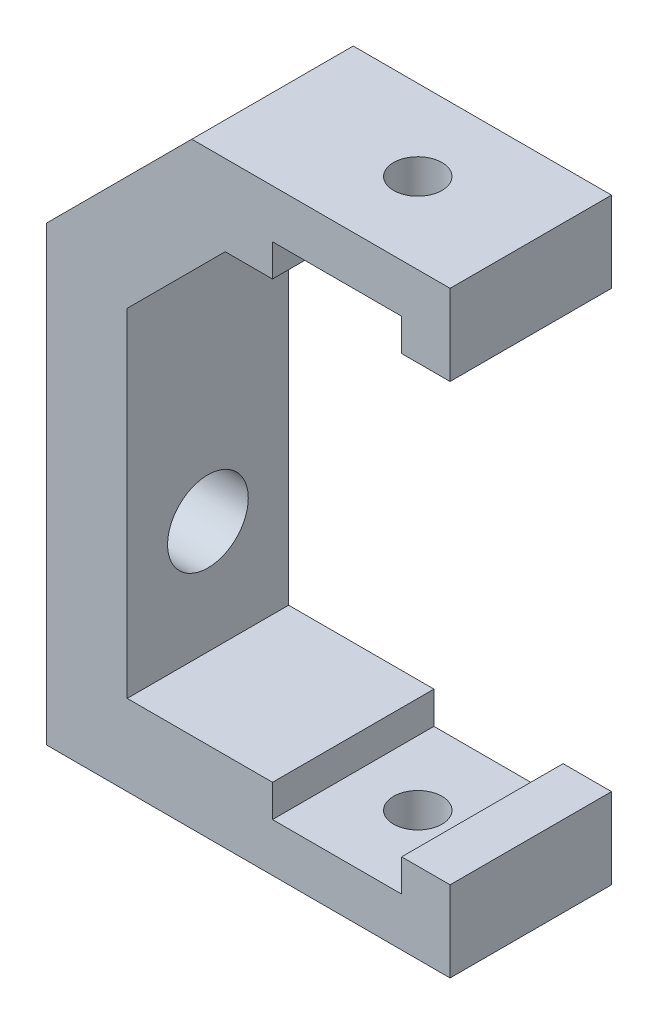
ISO-10303-21;
HEADER;
FILE_DESCRIPTION(('STEP AP214'),'2;1');
FILE_NAME('part.step','',(''),(''),'','','');
FILE_SCHEMA(('AUTOMOTIVE_DESIGN { 1 0 10303 214 1 1 1 1 }'));
ENDSEC;
DATA;
#1=APPLICATION_CONTEXT('core data for automotive mechanical design processes');
#2=APPLICATION_PROTOCOL_DEFINITION('international standard','automotive_design',2000,#1);
#3=PRODUCT_CONTEXT('',#1,'mechanical');
#4=PRODUCT('Part','Part','',(#3));
#5=PRODUCT_RELATED_PRODUCT_CATEGORY('part','',(#4));
#6=PRODUCT_DEFINITION_FORMATION('','',#4);
#7=PRODUCT_DEFINITION_CONTEXT('part definition',#1,'design');
#8=PRODUCT_DEFINITION('design','',#6,#7);
#9=PRODUCT_DEFINITION_SHAPE('','',#8);
#10=(LENGTH_UNIT() NAMED_UNIT(*) SI_UNIT(.MILLI.,.METRE.));
#11=(NAMED_UNIT(*) PLANE_ANGLE_UNIT() SI_UNIT($,.RADIAN.));
#12=(NAMED_UNIT(*) SI_UNIT($,.STERADIAN.) SOLID_ANGLE_UNIT());
#13=UNCERTAINTY_MEASURE_WITH_UNIT(LENGTH_MEASURE(1.E-05),#10,'distance_accuracy_value','');
#14=(GEOMETRIC_REPRESENTATION_CONTEXT(3) GLOBAL_UNCERTAINTY_ASSIGNED_CONTEXT((#13)) GLOBAL_UNIT_ASSIGNED_CONTEXT((#10,
#11,#12)) REPRESENTATION_CONTEXT('',''));
#15=CARTESIAN_POINT('',(0.,0.,0.));
#16=DIRECTION('',(0.,0.,1.));
#17=DIRECTION('',(1.,0.,0.));
#18=AXIS2_PLACEMENT_3D('',#15,#16,#17);
#19=CARTESIAN_POINT('',(25.,0.,5.));
#20=DIRECTION('',(0.,1.,0.));
#21=DIRECTION('',(-1.,0.,0.));
#22=AXIS2_PLACEMENT_3D('',#19,#20,#21);
#23=PLANE('',#22);
#24=CARTESIAN_POINT('',(18.,0.,0.));
#25=DIRECTION('',(0.,1.,0.));
#26=DIRECTION('',(-1.,0.,0.));
#27=AXIS2_PLACEMENT_3D('',#24,#25,#26);
#28=CIRCLE('',#27,1.5);
#29=CARTESIAN_POINT('',(16.5,0.,0.));
#30=VERTEX_POINT('',#29);
#31=EDGE_CURVE('E203',#30,#30,#28,.T.);
#32=ORIENTED_EDGE('',*,*,#31,.T.);
#33=EDGE_LOOP('',(#32));
#34=FACE_BOUND('',#33,.T.);
#35=DIRECTION('',(1.,0.,0.));
#36=VECTOR('',#35,1.);
#37=CARTESIAN_POINT('',(25.,0.,-5.));
#38=LINE('',#37,#36);
#39=CARTESIAN_POINT('',(0.,0.,-5.));
#40=VERTEX_POINT('',#39);
#41=CARTESIAN_POINT('',(25.,0.,-5.));
#42=VERTEX_POINT('',#41);
#43=EDGE_CURVE('E197',#40,#42,#38,.T.);
#44=ORIENTED_EDGE('',*,*,#43,.T.);
#45=DIRECTION('',(0.,0.,-1.));
#46=VECTOR('',#45,1.);
#47=CARTESIAN_POINT('',(25.,0.,5.));
#48=LINE('',#47,#46);
#49=CARTESIAN_POINT('',(25.,0.,5.));
#50=VERTEX_POINT('',#49);
#51=EDGE_CURVE('E11',#50,#42,#48,.T.);
#52=ORIENTED_EDGE('',*,*,#51,.F.);
#53=DIRECTION('',(1.,0.,0.));
#54=VECTOR('',#53,1.);
#55=CARTESIAN_POINT('',(25.,0.,5.));
#56=LINE('',#55,#54);
#57=CARTESIAN_POINT('',(0.,0.,5.));
#58=VERTEX_POINT('',#57);
#59=EDGE_CURVE('E232',#58,#50,#56,.T.);
#60=ORIENTED_EDGE('',*,*,#59,.F.);
#61=DIRECTION('',(0.,0.,-1.));
#62=VECTOR('',#61,1.);
#63=CARTESIAN_POINT('',(0.,0.,5.));
#64=LINE('',#63,#62);
#65=EDGE_CURVE('E194',#58,#40,#64,.T.);
#66=ORIENTED_EDGE('',*,*,#65,.T.);
#67=EDGE_LOOP('',(#44,#52,#60,#66));
#68=FACE_BOUND('',#67,.T.);
#69=ADVANCED_FACE('F39',(#34,#68),#23,.F.);
#70=CARTESIAN_POINT('',(25.,5.,5.));
#71=DIRECTION('',(-1.,0.,0.));
#72=DIRECTION('',(0.,-1.,0.));
#73=AXIS2_PLACEMENT_3D('',#70,#71,#72);
#74=PLANE('',#73);
#75=DIRECTION('',(0.,1.,0.));
#76=VECTOR('',#75,1.);
#77=CARTESIAN_POINT('',(25.,5.,-5.));
#78=LINE('',#77,#76);
#79=CARTESIAN_POINT('',(25.,5.,-5.));
#80=VERTEX_POINT('',#79);
#81=EDGE_CURVE('E199',#42,#80,#78,.T.);
#82=ORIENTED_EDGE('',*,*,#81,.T.);
#83=DIRECTION('',(0.,0.,-1.));
#84=VECTOR('',#83,1.);
#85=CARTESIAN_POINT('',(25.,5.,5.));
#86=LINE('',#85,#84);
#87=CARTESIAN_POINT('',(25.,5.,5.));
#88=VERTEX_POINT('',#87);
#89=EDGE_CURVE('E48',#88,#80,#86,.T.);
#90=ORIENTED_EDGE('',*,*,#89,.F.);
#91=DIRECTION('',(0.,1.,0.));
#92=VECTOR('',#91,1.);
#93=CARTESIAN_POINT('',(25.,5.,5.));
#94=LINE('',#93,#92);
#95=EDGE_CURVE('E128',#50,#88,#94,.T.);
#96=ORIENTED_EDGE('',*,*,#95,.F.);
#97=ORIENTED_EDGE('',*,*,#51,.T.);
#98=EDGE_LOOP('',(#82,#90,#96,#97));
#99=FACE_BOUND('',#98,.T.);
#100=ADVANCED_FACE('F346',(#99),#74,.F.);
#101=CARTESIAN_POINT('',(22.,5.,5.));
#102=DIRECTION('',(0.,-1.,0.));
#103=DIRECTION('',(0.,0.,-1.));
#104=AXIS2_PLACEMENT_3D('',#101,#102,#103);
#105=PLANE('',#104);
#106=DIRECTION('',(-1.,0.,0.));
#107=VECTOR('',#106,1.);
#108=CARTESIAN_POINT('',(22.,5.,-5.));
#109=LINE('',#108,#107);
#110=CARTESIAN_POINT('',(22.,5.,-5.));
#111=VERTEX_POINT('',#110);
#112=EDGE_CURVE('E201',#80,#111,#109,.T.);
#113=ORIENTED_EDGE('',*,*,#112,.T.);
#114=DIRECTION('',(0.,0.,-1.));
#115=VECTOR('',#114,1.);
#116=CARTESIAN_POINT('',(22.,5.,5.));
#117=LINE('',#116,#115);
#118=CARTESIAN_POINT('',(22.,5.,5.));
#119=VERTEX_POINT('',#118);
#120=EDGE_CURVE('E267',#119,#111,#117,.T.);
#121=ORIENTED_EDGE('',*,*,#120,.F.);
#122=DIRECTION('',(-1.,0.,0.));
#123=VECTOR('',#122,1.);
#124=CARTESIAN_POINT('',(22.,5.,5.));
#125=LINE('',#124,#123);
#126=EDGE_CURVE('E294',#88,#119,#125,.T.);
#127=ORIENTED_EDGE('',*,*,#126,.F.);
#128=ORIENTED_EDGE('',*,*,#89,.T.);
#129=EDGE_LOOP('',(#113,#121,#127,#128));
#130=FACE_BOUND('',#129,.T.);
#131=ADVANCED_FACE('F351',(#130),#105,.F.);
#132=CARTESIAN_POINT('',(22.,3.,5.));
#133=DIRECTION('',(1.,0.,0.));
#134=DIRECTION('',(0.,0.,-1.));
#135=AXIS2_PLACEMENT_3D('',#132,#133,#134);
#136=PLANE('',#135);
#137=DIRECTION('',(0.,-1.,0.));
#138=VECTOR('',#137,1.);
#139=CARTESIAN_POINT('',(22.,3.,-5.));
#140=LINE('',#139,#138);
#141=CARTESIAN_POINT('',(22.,3.,-5.));
#142=VERTEX_POINT('',#141);
#143=EDGE_CURVE('E202',#111,#142,#140,.T.);
#144=ORIENTED_EDGE('',*,*,#143,.T.);
#145=DIRECTION('',(0.,0.,-1.));
#146=VECTOR('',#145,1.);
#147=CARTESIAN_POINT('',(22.,3.,5.));
#148=LINE('',#147,#146);
#149=CARTESIAN_POINT('',(22.,3.,5.));
#150=VERTEX_POINT('',#149);
#151=EDGE_CURVE('E266',#150,#142,#148,.T.);
#152=ORIENTED_EDGE('',*,*,#151,.F.);
#153=DIRECTION('',(0.,-1.,0.));
#154=VECTOR('',#153,1.);
#155=CARTESIAN_POINT('',(22.,3.,5.));
#156=LINE('',#155,#154);
#157=EDGE_CURVE('E298',#119,#150,#156,.T.);
#158=ORIENTED_EDGE('',*,*,#157,.F.);
#159=ORIENTED_EDGE('',*,*,#120,.T.);
#160=EDGE_LOOP('',(#144,#152,#158,#159));
#161=FACE_BOUND('',#160,.T.);
#162=ADVANCED_FACE('F462',(#161),#136,.F.);
#163=CARTESIAN_POINT('',(14.,3.,5.));
#164=DIRECTION('',(0.,-1.,0.));
#165=DIRECTION('',(0.,0.,-1.));
#166=AXIS2_PLACEMENT_3D('',#163,#164,#165);
#167=PLANE('',#166);
#168=CARTESIAN_POINT('',(18.,3.,0.));
#169=DIRECTION('',(0.,-1.,0.));
#170=DIRECTION('',(0.,0.,-1.));
#171=AXIS2_PLACEMENT_3D('',#168,#169,#170);
#172=CIRCLE('',#171,1.5);
#173=CARTESIAN_POINT('',(18.,3.,-1.5));
#174=VERTEX_POINT('',#173);
#175=EDGE_CURVE('E278',#174,#174,#172,.T.);
#176=ORIENTED_EDGE('',*,*,#175,.T.);
#177=EDGE_LOOP('',(#176));
#178=FACE_BOUND('',#177,.T.);
#179=DIRECTION('',(-1.,0.,0.));
#180=VECTOR('',#179,1.);
#181=CARTESIAN_POINT('',(14.,3.,-5.));
#182=LINE('',#181,#180);
#183=CARTESIAN_POINT('',(14.,3.,-5.));
#184=VERTEX_POINT('',#183);
#185=EDGE_CURVE('E210',#142,#184,#182,.T.);
#186=ORIENTED_EDGE('',*,*,#185,.T.);
#187=DIRECTION('',(0.,0.,-1.));
#188=VECTOR('',#187,1.);
#189=CARTESIAN_POINT('',(14.,3.,5.));
#190=LINE('',#189,#188);
#191=CARTESIAN_POINT('',(14.,3.,5.));
#192=VERTEX_POINT('',#191);
#193=EDGE_CURVE('E263',#192,#184,#190,.T.);
#194=ORIENTED_EDGE('',*,*,#193,.F.);
#195=DIRECTION('',(-1.,0.,0.));
#196=VECTOR('',#195,1.);
#197=CARTESIAN_POINT('',(14.,3.,5.));
#198=LINE('',#197,#196);
#199=EDGE_CURVE('E297',#150,#192,#198,.T.);
#200=ORIENTED_EDGE('',*,*,#199,.F.);
#201=ORIENTED_EDGE('',*,*,#151,.T.);
#202=EDGE_LOOP('',(#186,#194,#200,#201));
#203=FACE_BOUND('',#202,.T.);
#204=ADVANCED_FACE('F457',(#178,#203),#167,.F.);
#205=CARTESIAN_POINT('',(14.,5.,5.));
#206=DIRECTION('',(-1.,0.,0.));
#207=DIRECTION('',(0.,0.,1.));
#208=AXIS2_PLACEMENT_3D('',#205,#206,#207);
#209=PLANE('',#208);
#210=DIRECTION('',(0.,1.,0.));
#211=VECTOR('',#210,1.);
#212=CARTESIAN_POINT('',(14.,5.,-5.));
#213=LINE('',#212,#211);
#214=CARTESIAN_POINT('',(14.,5.,-5.));
#215=VERTEX_POINT('',#214);
#216=EDGE_CURVE('E207',#184,#215,#213,.T.);
#217=ORIENTED_EDGE('',*,*,#216,.T.);
#218=DIRECTION('',(0.,0.,-1.));
#219=VECTOR('',#218,1.);
#220=CARTESIAN_POINT('',(14.,5.,5.));
#221=LINE('',#220,#219);
#222=CARTESIAN_POINT('',(14.,5.,5.));
#223=VERTEX_POINT('',#222);
#224=EDGE_CURVE('E257',#223,#215,#221,.T.);
#225=ORIENTED_EDGE('',*,*,#224,.F.);
#226=DIRECTION('',(0.,1.,0.));
#227=VECTOR('',#226,1.);
#228=CARTESIAN_POINT('',(14.,5.,5.));
#229=LINE('',#228,#227);
#230=EDGE_CURVE('E296',#192,#223,#229,.T.);
#231=ORIENTED_EDGE('',*,*,#230,.F.);
#232=ORIENTED_EDGE('',*,*,#193,.T.);
#233=EDGE_LOOP('',(#217,#225,#231,#232));
#234=FACE_BOUND('',#233,.T.);
#235=ADVANCED_FACE('F449',(#234),#209,.F.);
#236=CARTESIAN_POINT('',(5.,5.,5.));
#237=DIRECTION('',(0.,-1.,0.));
#238=DIRECTION('',(0.,0.,-1.));
#239=AXIS2_PLACEMENT_3D('',#236,#237,#238);
#240=PLANE('',#239);
#241=DIRECTION('',(-1.,0.,0.));
#242=VECTOR('',#241,1.);
#243=CARTESIAN_POINT('',(5.,5.,-5.));
#244=LINE('',#243,#242);
#245=CARTESIAN_POINT('',(5.,5.,-5.));
#246=VERTEX_POINT('',#245);
#247=EDGE_CURVE('E211',#215,#246,#244,.T.);
#248=ORIENTED_EDGE('',*,*,#247,.T.);
#249=DIRECTION('',(0.,0.,-1.));
#250=VECTOR('',#249,1.);
#251=CARTESIAN_POINT('',(5.,5.,5.));
#252=LINE('',#251,#250);
#253=CARTESIAN_POINT('',(5.,5.,5.));
#254=VERTEX_POINT('',#253);
#255=EDGE_CURVE('E260',#254,#246,#252,.T.);
#256=ORIENTED_EDGE('',*,*,#255,.F.);
#257=DIRECTION('',(-1.,0.,0.));
#258=VECTOR('',#257,1.);
#259=CARTESIAN_POINT('',(5.,5.,5.));
#260=LINE('',#259,#258);
#261=EDGE_CURVE('E302',#223,#254,#260,.T.);
#262=ORIENTED_EDGE('',*,*,#261,.F.);
#263=ORIENTED_EDGE('',*,*,#224,.T.);
#264=EDGE_LOOP('',(#248,#256,#262,#263));
#265=FACE_BOUND('',#264,.T.);
#266=ADVANCED_FACE('F444',(#265),#240,.F.);
#267=CARTESIAN_POINT('',(5.,25.9289321881346,5.));
#268=DIRECTION('',(-1.,0.,0.));
#269=DIRECTION('',(0.,-1.,0.));
#270=AXIS2_PLACEMENT_3D('',#267,#268,#269);
#271=PLANE('',#270);
#272=CARTESIAN_POINT('',(5.,12.,0.));
#273=DIRECTION('',(-1.,0.,0.));
#274=DIRECTION('',(0.,-1.,0.));
#275=AXIS2_PLACEMENT_3D('',#272,#273,#274);
#276=CIRCLE('',#275,2.5);
#277=CARTESIAN_POINT('',(5.,9.5,0.));
#278=VERTEX_POINT('',#277);
#279=EDGE_CURVE('E277',#278,#278,#276,.T.);
#280=ORIENTED_EDGE('',*,*,#279,.T.);
#281=EDGE_LOOP('',(#280));
#282=FACE_BOUND('',#281,.T.);
#283=DIRECTION('',(0.,1.,0.));
#284=VECTOR('',#283,1.);
#285=CARTESIAN_POINT('',(5.,25.9289321881346,-5.));
#286=LINE('',#285,#284);
#287=CARTESIAN_POINT('',(5.,25.9289321881346,-5.));
#288=VERTEX_POINT('',#287);
#289=EDGE_CURVE('E213',#246,#288,#286,.T.);
#290=ORIENTED_EDGE('',*,*,#289,.T.);
#291=DIRECTION('',(0.,0.,-1.));
#292=VECTOR('',#291,1.);
#293=CARTESIAN_POINT('',(5.,25.9289321881346,5.));
#294=LINE('',#293,#292);
#295=CARTESIAN_POINT('',(5.,25.9289321881346,5.));
#296=VERTEX_POINT('',#295);
#297=EDGE_CURVE('E255',#296,#288,#294,.T.);
#298=ORIENTED_EDGE('',*,*,#297,.F.);
#299=DIRECTION('',(0.,1.,0.));
#300=VECTOR('',#299,1.);
#301=CARTESIAN_POINT('',(5.,25.9289321881346,5.));
#302=LINE('',#301,#300);
#303=EDGE_CURVE('E303',#254,#296,#302,.T.);
#304=ORIENTED_EDGE('',*,*,#303,.F.);
#305=ORIENTED_EDGE('',*,*,#255,.T.);
#306=EDGE_LOOP('',(#290,#298,#304,#305));
#307=FACE_BOUND('',#306,.T.);
#308=ADVANCED_FACE('F436',(#282,#307),#271,.F.);
#309=CARTESIAN_POINT('',(11.0710678118653,32.,5.));
#310=DIRECTION('',(-0.707106781186556,0.707106781186539,0.));
#311=DIRECTION('',(-0.707106781186539,-0.707106781186556,0.));
#312=AXIS2_PLACEMENT_3D('',#309,#310,#311);
#313=PLANE('',#312);
#314=DIRECTION('',(0.707106781186539,0.707106781186556,0.));
#315=VECTOR('',#314,1.);
#316=CARTESIAN_POINT('',(11.0710678118653,32.,-5.));
#317=LINE('',#316,#315);
#318=CARTESIAN_POINT('',(11.0710678118653,32.,-5.));
#319=VERTEX_POINT('',#318);
#320=EDGE_CURVE('E214',#288,#319,#317,.T.);
#321=ORIENTED_EDGE('',*,*,#320,.T.);
#322=DIRECTION('',(0.,0.,-1.));
#323=VECTOR('',#322,1.);
#324=CARTESIAN_POINT('',(11.0710678118653,32.,5.));
#325=LINE('',#324,#323);
#326=CARTESIAN_POINT('',(11.0710678118653,32.,5.));
#327=VERTEX_POINT('',#326);
#328=EDGE_CURVE('E253',#327,#319,#325,.T.);
#329=ORIENTED_EDGE('',*,*,#328,.F.);
#330=DIRECTION('',(0.707106781186539,0.707106781186556,0.));
#331=VECTOR('',#330,1.);
#332=CARTESIAN_POINT('',(11.0710678118653,32.,5.));
#333=LINE('',#332,#331);
#334=EDGE_CURVE('E308',#296,#327,#333,.T.);
#335=ORIENTED_EDGE('',*,*,#334,.F.);
#336=ORIENTED_EDGE('',*,*,#297,.T.);
#337=EDGE_LOOP('',(#321,#329,#335,#336));
#338=FACE_BOUND('',#337,.T.);
#339=ADVANCED_FACE('F430',(#338),#313,.F.);
#340=CARTESIAN_POINT('',(14.,32.,5.));
#341=DIRECTION('',(0.,1.,0.));
#342=DIRECTION('',(0.,0.,1.));
#343=AXIS2_PLACEMENT_3D('',#340,#341,#342);
#344=PLANE('',#343);
#345=DIRECTION('',(1.,0.,0.));
#346=VECTOR('',#345,1.);
#347=CARTESIAN_POINT('',(14.,32.,-5.));
#348=LINE('',#347,#346);
#349=CARTESIAN_POINT('',(14.,32.,-5.));
#350=VERTEX_POINT('',#349);
#351=EDGE_CURVE('E220',#319,#350,#348,.T.);
#352=ORIENTED_EDGE('',*,*,#351,.T.);
#353=DIRECTION('',(0.,0.,-1.));
#354=VECTOR('',#353,1.);
#355=CARTESIAN_POINT('',(14.,32.,5.));
#356=LINE('',#355,#354);
#357=CARTESIAN_POINT('',(14.,32.,5.));
#358=VERTEX_POINT('',#357);
#359=EDGE_CURVE('E249',#358,#350,#356,.T.);
#360=ORIENTED_EDGE('',*,*,#359,.F.);
#361=DIRECTION('',(1.,0.,0.));
#362=VECTOR('',#361,1.);
#363=CARTESIAN_POINT('',(14.,32.,5.));
#364=LINE('',#363,#362);
#365=EDGE_CURVE('E306',#327,#358,#364,.T.);
#366=ORIENTED_EDGE('',*,*,#365,.F.);
#367=ORIENTED_EDGE('',*,*,#328,.T.);
#368=EDGE_LOOP('',(#352,#360,#366,#367));
#369=FACE_BOUND('',#368,.T.);
#370=ADVANCED_FACE('F416',(#369),#344,.F.);
#371=CARTESIAN_POINT('',(14.,34.,5.));
#372=DIRECTION('',(-1.,0.,0.));
#373=DIRECTION('',(0.,0.,1.));
#374=AXIS2_PLACEMENT_3D('',#371,#372,#373);
#375=PLANE('',#374);
#376=DIRECTION('',(0.,1.,0.));
#377=VECTOR('',#376,1.);
#378=CARTESIAN_POINT('',(14.,34.,-5.));
#379=LINE('',#378,#377);
#380=CARTESIAN_POINT('',(14.,34.,-5.));
#381=VERTEX_POINT('',#380);
#382=EDGE_CURVE('E218',#350,#381,#379,.T.);
#383=ORIENTED_EDGE('',*,*,#382,.T.);
#384=DIRECTION('',(0.,0.,-1.));
#385=VECTOR('',#384,1.);
#386=CARTESIAN_POINT('',(14.,34.,5.));
#387=LINE('',#386,#385);
#388=CARTESIAN_POINT('',(14.,34.,5.));
#389=VERTEX_POINT('',#388);
#390=EDGE_CURVE('E241',#389,#381,#387,.T.);
#391=ORIENTED_EDGE('',*,*,#390,.F.);
#392=DIRECTION('',(0.,1.,0.));
#393=VECTOR('',#392,1.);
#394=CARTESIAN_POINT('',(14.,34.,5.));
#395=LINE('',#394,#393);
#396=EDGE_CURVE('E309',#358,#389,#395,.T.);
#397=ORIENTED_EDGE('',*,*,#396,.F.);
#398=ORIENTED_EDGE('',*,*,#359,.T.);
#399=EDGE_LOOP('',(#383,#391,#397,#398));
#400=FACE_BOUND('',#399,.T.);
#401=ADVANCED_FACE('F413',(#400),#375,.F.);
#402=CARTESIAN_POINT('',(22.,34.,5.));
#403=DIRECTION('',(0.,1.,0.));
#404=DIRECTION('',(-1.,0.,0.));
#405=AXIS2_PLACEMENT_3D('',#402,#403,#404);
#406=PLANE('',#405);
#407=CARTESIAN_POINT('',(18.,34.,0.));
#408=DIRECTION('',(0.,1.,0.));
#409=DIRECTION('',(-1.,0.,0.));
#410=AXIS2_PLACEMENT_3D('',#407,#408,#409);
#411=CIRCLE('',#410,1.5);
#412=CARTESIAN_POINT('',(16.5,34.,0.));
#413=VERTEX_POINT('',#412);
#414=EDGE_CURVE('E274',#413,#413,#411,.T.);
#415=ORIENTED_EDGE('',*,*,#414,.T.);
#416=EDGE_LOOP('',(#415));
#417=FACE_BOUND('',#416,.T.);
#418=DIRECTION('',(1.,0.,0.));
#419=VECTOR('',#418,1.);
#420=CARTESIAN_POINT('',(22.,34.,-5.));
#421=LINE('',#420,#419);
#422=CARTESIAN_POINT('',(22.,34.,-5.));
#423=VERTEX_POINT('',#422);
#424=EDGE_CURVE('E222',#381,#423,#421,.T.);
#425=ORIENTED_EDGE('',*,*,#424,.T.);
#426=DIRECTION('',(0.,0.,-1.));
#427=VECTOR('',#426,1.);
#428=CARTESIAN_POINT('',(22.,34.,5.));
#429=LINE('',#428,#427);
#430=CARTESIAN_POINT('',(22.,34.,5.));
#431=VERTEX_POINT('',#430);
#432=EDGE_CURVE('E244',#431,#423,#429,.T.);
#433=ORIENTED_EDGE('',*,*,#432,.F.);
#434=DIRECTION('',(1.,0.,0.));
#435=VECTOR('',#434,1.);
#436=CARTESIAN_POINT('',(22.,34.,5.));
#437=LINE('',#436,#435);
#438=EDGE_CURVE('E315',#389,#431,#437,.T.);
#439=ORIENTED_EDGE('',*,*,#438,.F.);
#440=ORIENTED_EDGE('',*,*,#390,.T.);
#441=EDGE_LOOP('',(#425,#433,#439,#440));
#442=FACE_BOUND('',#441,.T.);
#443=ADVANCED_FACE('F409',(#417,#442),#406,.F.);
#444=CARTESIAN_POINT('',(22.,32.,5.));
#445=DIRECTION('',(1.,0.,0.));
#446=DIRECTION('',(0.,1.,0.));
#447=AXIS2_PLACEMENT_3D('',#444,#445,#446);
#448=PLANE('',#447);
#449=DIRECTION('',(0.,-1.,0.));
#450=VECTOR('',#449,1.);
#451=CARTESIAN_POINT('',(22.,32.,-5.));
#452=LINE('',#451,#450);
#453=CARTESIAN_POINT('',(22.,32.,-5.));
#454=VERTEX_POINT('',#453);
#455=EDGE_CURVE('E224',#423,#454,#452,.T.);
#456=ORIENTED_EDGE('',*,*,#455,.T.);
#457=DIRECTION('',(0.,0.,-1.));
#458=VECTOR('',#457,1.);
#459=CARTESIAN_POINT('',(22.,32.,5.));
#460=LINE('',#459,#458);
#461=CARTESIAN_POINT('',(22.,32.,5.));
#462=VERTEX_POINT('',#461);
#463=EDGE_CURVE('E239',#462,#454,#460,.T.);
#464=ORIENTED_EDGE('',*,*,#463,.F.);
#465=DIRECTION('',(0.,-1.,0.));
#466=VECTOR('',#465,1.);
#467=CARTESIAN_POINT('',(22.,32.,5.));
#468=LINE('',#467,#466);
#469=EDGE_CURVE('E314',#431,#462,#468,.T.);
#470=ORIENTED_EDGE('',*,*,#469,.F.);
#471=ORIENTED_EDGE('',*,*,#432,.T.);
#472=EDGE_LOOP('',(#456,#464,#470,#471));
#473=FACE_BOUND('',#472,.T.);
#474=ADVANCED_FACE('F398',(#473),#448,.F.);
#475=CARTESIAN_POINT('',(25.,32.,5.));
#476=DIRECTION('',(0.,1.,0.));
#477=DIRECTION('',(0.,0.,1.));
#478=AXIS2_PLACEMENT_3D('',#475,#476,#477);
#479=PLANE('',#478);
#480=DIRECTION('',(1.,0.,0.));
#481=VECTOR('',#480,1.);
#482=CARTESIAN_POINT('',(25.,32.,-5.));
#483=LINE('',#482,#481);
#484=CARTESIAN_POINT('',(25.,32.,-5.));
#485=VERTEX_POINT('',#484);
#486=EDGE_CURVE('E223',#454,#485,#483,.T.);
#487=ORIENTED_EDGE('',*,*,#486,.T.);
#488=DIRECTION('',(0.,0.,-1.));
#489=VECTOR('',#488,1.);
#490=CARTESIAN_POINT('',(25.,32.,5.));
#491=LINE('',#490,#489);
#492=CARTESIAN_POINT('',(25.,32.,5.));
#493=VERTEX_POINT('',#492);
#494=EDGE_CURVE('E237',#493,#485,#491,.T.);
#495=ORIENTED_EDGE('',*,*,#494,.F.);
#496=DIRECTION('',(1.,0.,0.));
#497=VECTOR('',#496,1.);
#498=CARTESIAN_POINT('',(25.,32.,5.));
#499=LINE('',#498,#497);
#500=EDGE_CURVE('E316',#462,#493,#499,.T.);
#501=ORIENTED_EDGE('',*,*,#500,.F.);
#502=ORIENTED_EDGE('',*,*,#463,.T.);
#503=EDGE_LOOP('',(#487,#495,#501,#502));
#504=FACE_BOUND('',#503,.T.);
#505=ADVANCED_FACE('F325',(#504),#479,.F.);
#506=CARTESIAN_POINT('',(25.,37.,5.));
#507=DIRECTION('',(-1.,0.,0.));
#508=DIRECTION('',(0.,-1.,0.));
#509=AXIS2_PLACEMENT_3D('',#506,#507,#508);
#510=PLANE('',#509);
#511=DIRECTION('',(0.,1.,0.));
#512=VECTOR('',#511,1.);
#513=CARTESIAN_POINT('',(25.,37.,-5.));
#514=LINE('',#513,#512);
#515=CARTESIAN_POINT('',(25.,37.,-5.));
#516=VERTEX_POINT('',#515);
#517=EDGE_CURVE('E229',#485,#516,#514,.T.);
#518=ORIENTED_EDGE('',*,*,#517,.T.);
#519=DIRECTION('',(0.,0.,-1.));
#520=VECTOR('',#519,1.);
#521=CARTESIAN_POINT('',(25.,37.,5.));
#522=LINE('',#521,#520);
#523=CARTESIAN_POINT('',(25.,37.,5.));
#524=VERTEX_POINT('',#523);
#525=EDGE_CURVE('E187',#524,#516,#522,.T.);
#526=ORIENTED_EDGE('',*,*,#525,.F.);
#527=DIRECTION('',(0.,1.,0.));
#528=VECTOR('',#527,1.);
#529=CARTESIAN_POINT('',(25.,37.,5.));
#530=LINE('',#529,#528);
#531=EDGE_CURVE('E178',#493,#524,#530,.T.);
#532=ORIENTED_EDGE('',*,*,#531,.F.);
#533=ORIENTED_EDGE('',*,*,#494,.T.);
#534=EDGE_LOOP('',(#518,#526,#532,#533));
#535=FACE_BOUND('',#534,.T.);
#536=ADVANCED_FACE('F326',(#535),#510,.F.);
#537=CARTESIAN_POINT('',(8.99999999999977,37.,5.));
#538=DIRECTION('',(0.,-1.,0.));
#539=DIRECTION('',(0.,0.,-1.));
#540=AXIS2_PLACEMENT_3D('',#537,#538,#539);
#541=PLANE('',#540);
#542=CARTESIAN_POINT('',(18.,37.,0.));
#543=DIRECTION('',(0.,-1.,0.));
#544=DIRECTION('',(0.,0.,-1.));
#545=AXIS2_PLACEMENT_3D('',#542,#543,#544);
#546=CIRCLE('',#545,1.5);
#547=CARTESIAN_POINT('',(18.,37.,-1.5));
#548=VERTEX_POINT('',#547);
#549=EDGE_CURVE('E272',#548,#548,#546,.T.);
#550=ORIENTED_EDGE('',*,*,#549,.T.);
#551=EDGE_LOOP('',(#550));
#552=FACE_BOUND('',#551,.T.);
#553=DIRECTION('',(-1.,0.,0.));
#554=VECTOR('',#553,1.);
#555=CARTESIAN_POINT('',(8.99999999999977,37.,-5.));
#556=LINE('',#555,#554);
#557=CARTESIAN_POINT('',(8.99999999999977,37.,-5.));
#558=VERTEX_POINT('',#557);
#559=EDGE_CURVE('E189',#516,#558,#556,.T.);
#560=ORIENTED_EDGE('',*,*,#559,.T.);
#561=DIRECTION('',(0.,0.,-1.));
#562=VECTOR('',#561,1.);
#563=CARTESIAN_POINT('',(8.99999999999977,37.,5.));
#564=LINE('',#563,#562);
#565=CARTESIAN_POINT('',(8.99999999999977,37.,5.));
#566=VERTEX_POINT('',#565);
#567=EDGE_CURVE('E184',#566,#558,#564,.T.);
#568=ORIENTED_EDGE('',*,*,#567,.F.);
#569=DIRECTION('',(-1.,0.,0.));
#570=VECTOR('',#569,1.);
#571=CARTESIAN_POINT('',(8.99999999999977,37.,5.));
#572=LINE('',#571,#570);
#573=EDGE_CURVE('E172',#524,#566,#572,.T.);
#574=ORIENTED_EDGE('',*,*,#573,.F.);
#575=ORIENTED_EDGE('',*,*,#525,.T.);
#576=EDGE_LOOP('',(#560,#568,#574,#575));
#577=FACE_BOUND('',#576,.T.);
#578=ADVANCED_FACE('F183',(#552,#577),#541,.F.);
#579=CARTESIAN_POINT('',(0.,28.,5.));
#580=DIRECTION('',(0.707106781186556,-0.707106781186539,0.));
#581=DIRECTION('',(0.707106781186539,0.707106781186556,0.));
#582=AXIS2_PLACEMENT_3D('',#579,#580,#581);
#583=PLANE('',#582);
#584=DIRECTION('',(-0.707106781186539,-0.707106781186556,0.));
#585=VECTOR('',#584,1.);
#586=CARTESIAN_POINT('',(0.,28.,-5.));
#587=LINE('',#586,#585);
#588=CARTESIAN_POINT('',(0.,28.,-5.));
#589=VERTEX_POINT('',#588);
#590=EDGE_CURVE('E118',#558,#589,#587,.T.);
#591=ORIENTED_EDGE('',*,*,#590,.T.);
#592=DIRECTION('',(0.,0.,-1.));
#593=VECTOR('',#592,1.);
#594=CARTESIAN_POINT('',(0.,28.,5.));
#595=LINE('',#594,#593);
#596=CARTESIAN_POINT('',(0.,28.,5.));
#597=VERTEX_POINT('',#596);
#598=EDGE_CURVE('E190',#597,#589,#595,.T.);
#599=ORIENTED_EDGE('',*,*,#598,.F.);
#600=DIRECTION('',(-0.707106781186539,-0.707106781186556,0.));
#601=VECTOR('',#600,1.);
#602=CARTESIAN_POINT('',(0.,28.,5.));
#603=LINE('',#602,#601);
#604=EDGE_CURVE('E177',#566,#597,#603,.T.);
#605=ORIENTED_EDGE('',*,*,#604,.F.);
#606=ORIENTED_EDGE('',*,*,#567,.T.);
#607=EDGE_LOOP('',(#591,#599,#605,#606));
#608=FACE_BOUND('',#607,.T.);
#609=ADVANCED_FACE('F191',(#608),#583,.F.);
#610=CARTESIAN_POINT('',(0.,0.,5.));
#611=DIRECTION('',(1.,0.,0.));
#612=DIRECTION('',(0.,0.,-1.));
#613=AXIS2_PLACEMENT_3D('',#610,#611,#612);
#614=PLANE('',#613);
#615=CARTESIAN_POINT('',(0.,12.,0.));
#616=DIRECTION('',(1.,0.,0.));
#617=DIRECTION('',(0.,0.,-1.));
#618=AXIS2_PLACEMENT_3D('',#615,#616,#617);
#619=CIRCLE('',#618,2.5);
#620=CARTESIAN_POINT('',(0.,12.,-2.5));
#621=VERTEX_POINT('',#620);
#622=EDGE_CURVE('E45',#621,#621,#619,.T.);
#623=ORIENTED_EDGE('',*,*,#622,.T.);
#624=EDGE_LOOP('',(#623));
#625=FACE_BOUND('',#624,.T.);
#626=DIRECTION('',(0.,-1.,0.));
#627=VECTOR('',#626,1.);
#628=CARTESIAN_POINT('',(0.,0.,-5.));
#629=LINE('',#628,#627);
#630=EDGE_CURVE('E122',#589,#40,#629,.T.);
#631=ORIENTED_EDGE('',*,*,#630,.T.);
#632=ORIENTED_EDGE('',*,*,#65,.F.);
#633=DIRECTION('',(0.,-1.,0.));
#634=VECTOR('',#633,1.);
#635=CARTESIAN_POINT('',(0.,0.,5.));
#636=LINE('',#635,#634);
#637=EDGE_CURVE('E60',#597,#58,#636,.T.);
#638=ORIENTED_EDGE('',*,*,#637,.F.);
#639=ORIENTED_EDGE('',*,*,#598,.T.);
#640=EDGE_LOOP('',(#631,#632,#638,#639));
#641=FACE_BOUND('',#640,.T.);
#642=ADVANCED_FACE('F331',(#625,#641),#614,.F.);
#643=CARTESIAN_POINT('',(0.,0.,5.));
#644=DIRECTION('',(0.,0.,-1.));
#645=DIRECTION('',(-1.,0.,0.));
#646=AXIS2_PLACEMENT_3D('',#643,#644,#645);
#647=PLANE('',#646);
#648=ORIENTED_EDGE('',*,*,#59,.T.);
#649=ORIENTED_EDGE('',*,*,#95,.T.);
#650=ORIENTED_EDGE('',*,*,#126,.T.);
#651=ORIENTED_EDGE('',*,*,#157,.T.);
#652=ORIENTED_EDGE('',*,*,#199,.T.);
#653=ORIENTED_EDGE('',*,*,#230,.T.);
#654=ORIENTED_EDGE('',*,*,#261,.T.);
#655=ORIENTED_EDGE('',*,*,#303,.T.);
#656=ORIENTED_EDGE('',*,*,#334,.T.);
#657=ORIENTED_EDGE('',*,*,#365,.T.);
#658=ORIENTED_EDGE('',*,*,#396,.T.);
#659=ORIENTED_EDGE('',*,*,#438,.T.);
#660=ORIENTED_EDGE('',*,*,#469,.T.);
#661=ORIENTED_EDGE('',*,*,#500,.T.);
#662=ORIENTED_EDGE('',*,*,#531,.T.);
#663=ORIENTED_EDGE('',*,*,#573,.T.);
#664=ORIENTED_EDGE('',*,*,#604,.T.);
#665=ORIENTED_EDGE('',*,*,#637,.T.);
#666=EDGE_LOOP('',(#648,#649,#650,#651,#652,#653,#654,#655,#656,#657,#658,#659,#660,#661,#662,
#663,#664,#665));
#667=FACE_BOUND('',#666,.T.);
#668=ADVANCED_FACE('F171',(#667),#647,.F.);
#669=CARTESIAN_POINT('',(0.,0.,-5.));
#670=DIRECTION('',(0.,0.,-1.));
#671=DIRECTION('',(-1.,0.,0.));
#672=AXIS2_PLACEMENT_3D('',#669,#670,#671);
#673=PLANE('',#672);
#674=ORIENTED_EDGE('',*,*,#43,.F.);
#675=ORIENTED_EDGE('',*,*,#630,.F.);
#676=ORIENTED_EDGE('',*,*,#590,.F.);
#677=ORIENTED_EDGE('',*,*,#559,.F.);
#678=ORIENTED_EDGE('',*,*,#517,.F.);
#679=ORIENTED_EDGE('',*,*,#486,.F.);
#680=ORIENTED_EDGE('',*,*,#455,.F.);
#681=ORIENTED_EDGE('',*,*,#424,.F.);
#682=ORIENTED_EDGE('',*,*,#382,.F.);
#683=ORIENTED_EDGE('',*,*,#351,.F.);
#684=ORIENTED_EDGE('',*,*,#320,.F.);
#685=ORIENTED_EDGE('',*,*,#289,.F.);
#686=ORIENTED_EDGE('',*,*,#247,.F.);
#687=ORIENTED_EDGE('',*,*,#216,.F.);
#688=ORIENTED_EDGE('',*,*,#185,.F.);
#689=ORIENTED_EDGE('',*,*,#143,.F.);
#690=ORIENTED_EDGE('',*,*,#112,.F.);
#691=ORIENTED_EDGE('',*,*,#81,.F.);
#692=EDGE_LOOP('',(#674,#675,#676,#677,#678,#679,#680,#681,#682,#683,#684,#685,#686,#687,#688,
#689,#690,#691));
#693=FACE_BOUND('',#692,.T.);
#694=ADVANCED_FACE('F328',(#693),#673,.T.);
#695=CARTESIAN_POINT('',(18.0000000000001,134.,0.));
#696=DIRECTION('',(0.,-1.,0.));
#697=DIRECTION('',(1.,0.,0.));
#698=AXIS2_PLACEMENT_3D('',#695,#696,#697);
#699=CYLINDRICAL_SURFACE('',#698,1.5);
#700=ORIENTED_EDGE('',*,*,#549,.F.);
#701=EDGE_LOOP('',(#700));
#702=FACE_BOUND('',#701,.T.);
#703=ORIENTED_EDGE('',*,*,#414,.F.);
#704=EDGE_LOOP('',(#703));
#705=FACE_BOUND('',#704,.T.);
#706=ADVANCED_FACE('F363',(#702,#705),#699,.F.);
#707=ORIENTED_EDGE('',*,*,#175,.F.);
#708=EDGE_LOOP('',(#707));
#709=FACE_BOUND('',#708,.T.);
#710=ORIENTED_EDGE('',*,*,#31,.F.);
#711=EDGE_LOOP('',(#710));
#712=FACE_BOUND('',#711,.T.);
#713=ADVANCED_FACE('F359',(#709,#712),#699,.F.);
#714=CARTESIAN_POINT('',(-95.,12.,0.));
#715=DIRECTION('',(1.,0.,0.));
#716=DIRECTION('',(0.,1.,0.));
#717=AXIS2_PLACEMENT_3D('',#714,#715,#716);
#718=CYLINDRICAL_SURFACE('',#717,2.5);
#719=ORIENTED_EDGE('',*,*,#622,.F.);
#720=EDGE_LOOP('',(#719));
#721=FACE_BOUND('',#720,.T.);
#722=ORIENTED_EDGE('',*,*,#279,.F.);
#723=EDGE_LOOP('',(#722));
#724=FACE_BOUND('',#723,.T.);
#725=ADVANCED_FACE('F360',(#721,#724),#718,.F.);
#726=CLOSED_SHELL('',(#69,#100,#131,#162,#204,#235,#266,#308,#339,#370,#401,#443,#474,#505,#536,
#578,#609,#642,#668,#694,#706,#713,#725));
#727=MANIFOLD_SOLID_BREP('B2',#726);
#728=ADVANCED_BREP_SHAPE_REPRESENTATION('',(#18,#727),#14);
#729=SHAPE_DEFINITION_REPRESENTATION(#9,#728);
ENDSEC;
END-ISO-10303-21;
